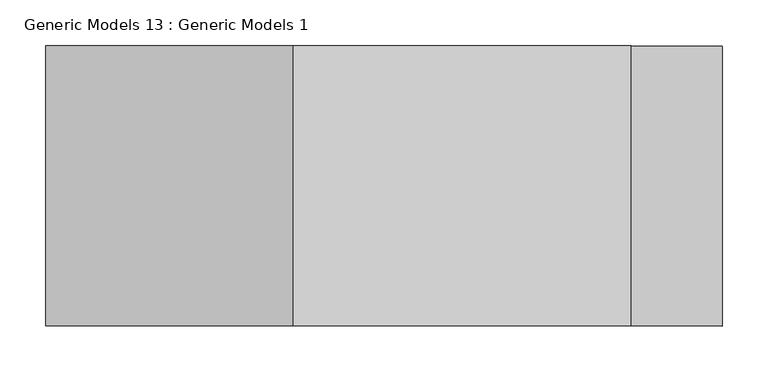
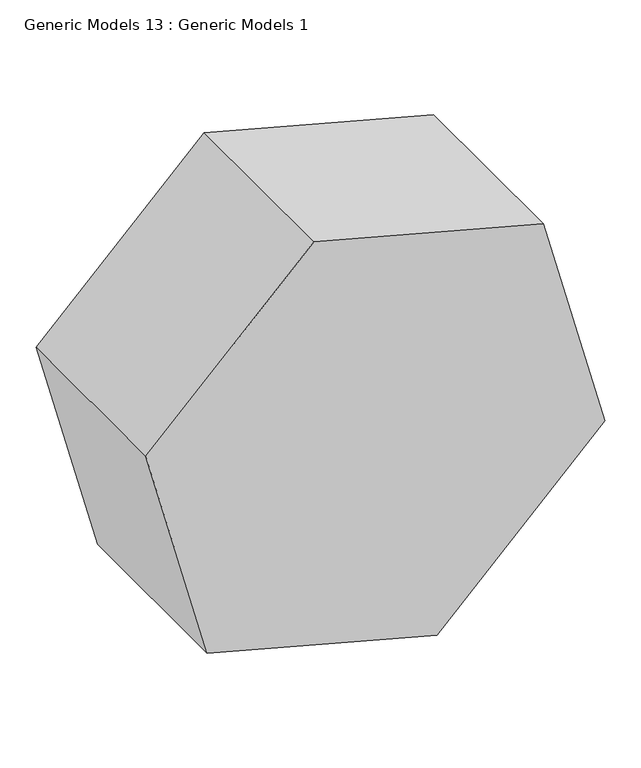
"""IFC4 building model written with IfcOpenShell, lengths in millimetres: proxy geometry, Generic Models 13 : Generic Models 1."""

from ifc_helpers import new_model, si_unit, frame, origin, place, context, project, spatial, polyline, outline, extrude, source, transform, mapped, element, save


def generic_models_13_generic_models_1_344792cf(model_context):
    return source(origin(), model_context, "Body", "SweptSolid", [
        extrude(outline(polyline([(904.7566299, 4249.8198357), (1003.366686, 3881.8020959), (733.9590024, 3612.3944123), (365.9412626, 3711.0044685), (267.3312064, 4079.0222083), (536.73889, 4348.4298919), (904.7566299, 4249.8198357)])), frame((0.0, -9086.6225464, 0.0), z_axis=(0.0, 1.0, 0.0), x_axis=(0.0, 0.0, 1.0)), (0.0, 0.0, 1.0), 304.8),
    ])


if __name__ == "__main__":
    model = new_model("IFC4")
    model_context = context("Model", 3, world=origin())
    ifc_project = project(units=[si_unit("LENGTHUNIT", "METRE", prefix="MILLI")], contexts=[model_context])
    site = spatial("IfcSite", under=ifc_project)
    building = spatial("IfcBuilding", under=site)
    placement = place(None, origin())
    generic_models_13_generic_models_1_shape = generic_models_13_generic_models_1_344792cf(model_context)
    element("IfcBuildingElementProxy", 1, Name="Generic Models 13 : Generic Models 1", ObjectType="Generic Models 13 : Generic Models 1", at=placement, inside=building, context=model_context, shape_type="MappedRepresentation", body=[
        mapped(generic_models_13_generic_models_1_shape, transform((0.0, 0.0, 0.0), x_axis=(1.0, 0.0, 0.0), y_axis=(0.0, 1.0, 0.0), z_axis=(0.0, 0.0, 1.0))),
    ])
    save(model, "model.ifc")

# Revit data of these elements
# Element 1 (IfcBuildingElementProxy, "Generic Models 13 : Generic Models 1")
#   Materials on its faces: "Carpet (1)"
# Materials
#   "Carpet (1)": class "Carpet", colour RGB 124 80 67, transparency 0, Description = "Interior finish", Cost = 0
